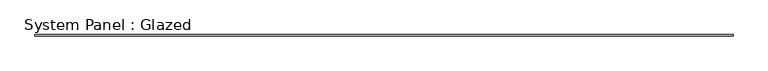
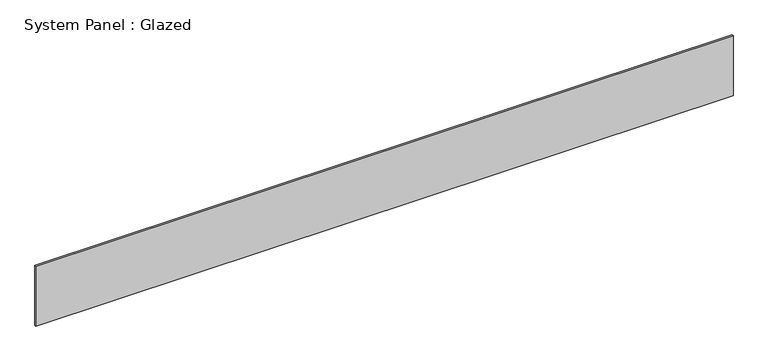
"""IFC4 building model written with IfcOpenShell, lengths in millimetres: plate geometry, System Panel : Glazed."""

from ifc_helpers import new_model, si_unit, origin, origin_with_axes, place, context, project, spatial, polyline, outline, extrude, source, transform, mapped, element, save


def system_panel_glazed_c82e1c3c(model_context):
    return source(origin(), model_context, "Body", "SweptSolid", [
        extrude(outline(polyline([(6367.6994619, 19.05), (-6367.6994619, 19.05), (-6367.6994619, 44.45), (6367.6994619, 44.45), (6367.6994619, 19.05)])), origin_with_axes(), (0.0, 0.0, 1.0), 1155.7),
    ])


if __name__ == "__main__":
    model = new_model("IFC4")
    model_context = context("Model", 3, world=origin())
    ifc_project = project(units=[si_unit("LENGTHUNIT", "METRE", prefix="MILLI")], contexts=[model_context])
    site = spatial("IfcSite", under=ifc_project)
    building = spatial("IfcBuilding", under=site)
    placement = place(None, origin())
    system_panel_glazed_shape = system_panel_glazed_c82e1c3c(model_context)
    element("IfcPlate", 1, ObjectType="System Panel : Glazed", at=placement, inside=building, context=model_context, shape_type="MappedRepresentation", body=[
        mapped(system_panel_glazed_shape, transform((0.0, 0.0, 0.0), x_axis=(1.0, 0.0, 0.0), y_axis=(0.0, 1.0, 0.0), z_axis=(0.0, 0.0, 1.0))),
    ])
    save(model, "model.ifc")

# Revit data of these elements
# Type "System Panel : Glazed"
#   Construction Type Id = "GSP4R"
#   Analytic Construction = "1/8 in Pilkington single glazing"
#   Visual Light Transmittance = 0.9
#   Solar Heat Gain Coefficient = 0.86
#   Heat Transfer Coefficient (U) = 1.18115 BTU/(h·ft²·°F)
# Element 1 (IfcPlate, "System Panel : Glazed")
#   Materials on its faces: "Glass"
# Materials
#   "Glass": class "Glass", colour RGB 0 128 192, transparency 0.75, Description = "Soda Lime Glass", Cost = 0
